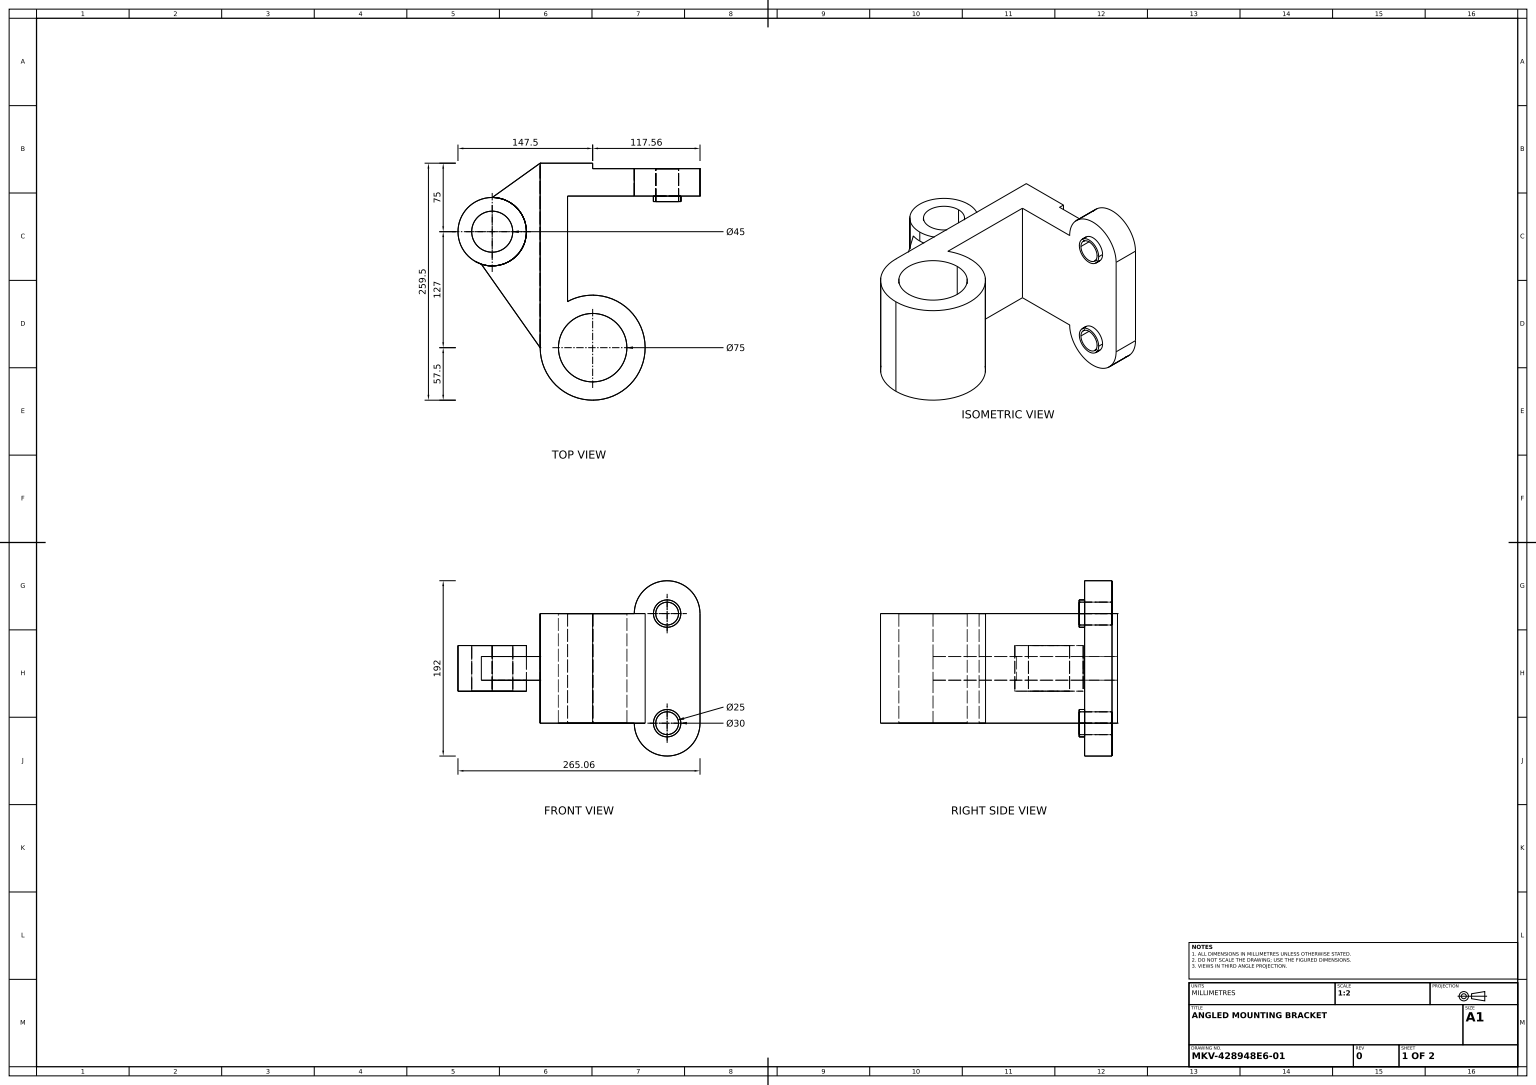
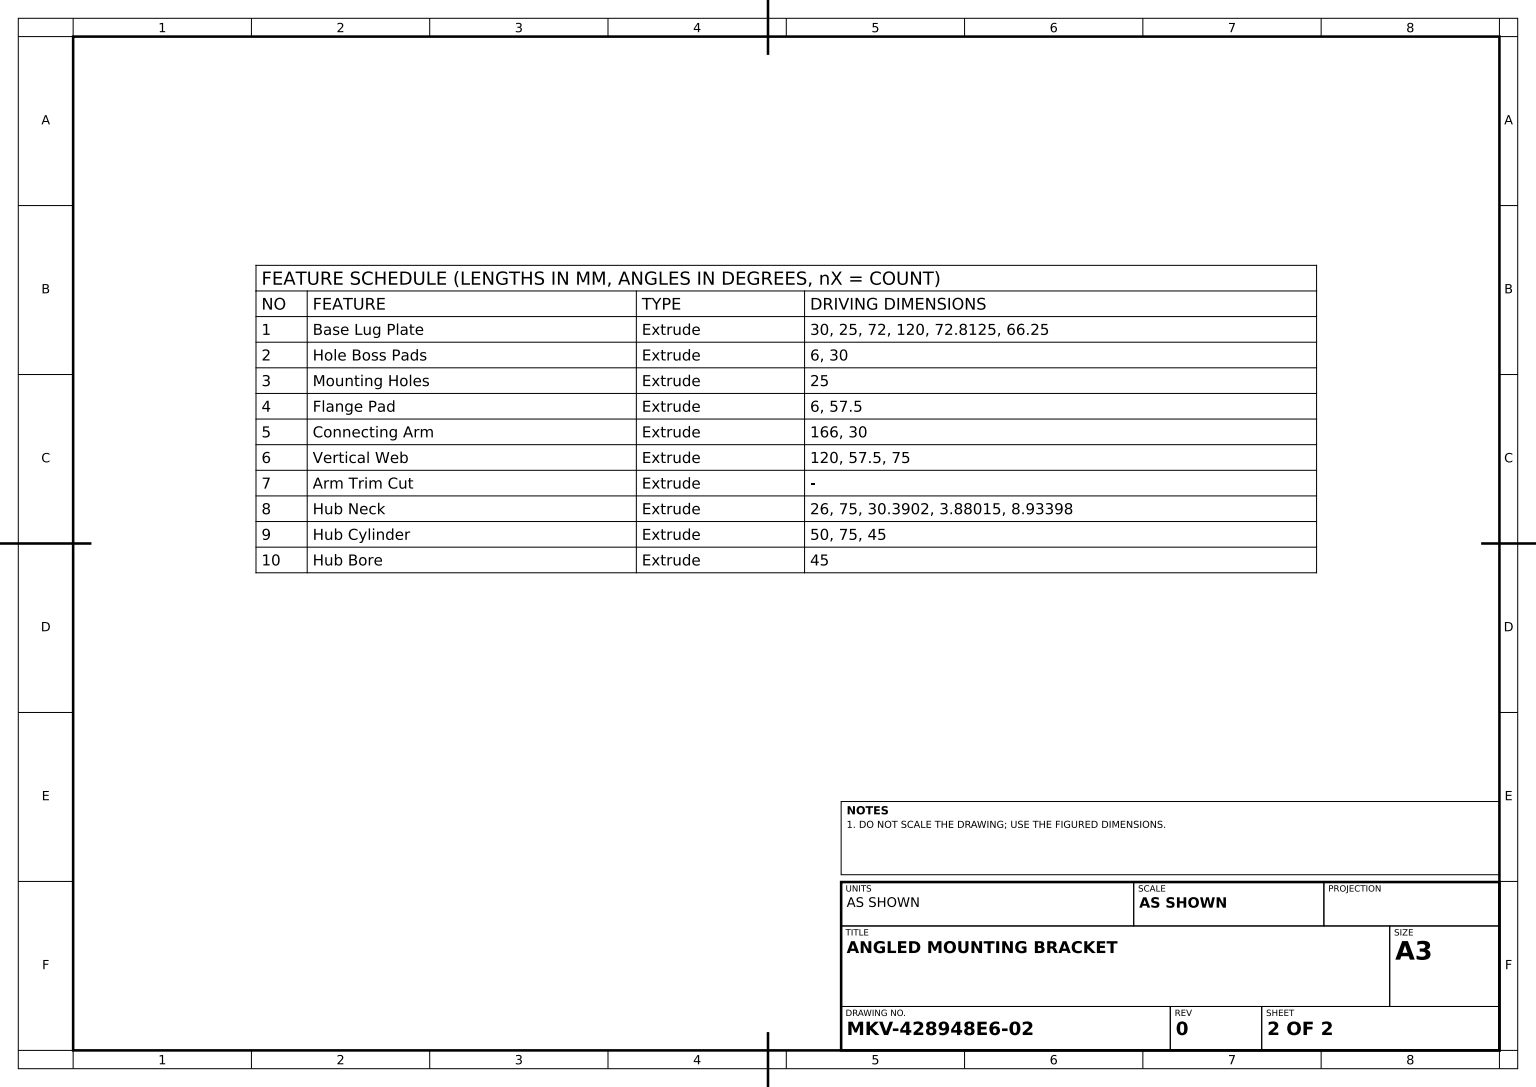
from build123d import *

# Parameters (mm, degrees)
BASE_PLATE_PROFILE_SKETCH_R = 12.5
BASE_LUG_PLATE_DEPTH        = 30
HOLE_BOSS_SKETCH_R          = 15
HOLE_BOSS_PADS_DEPTH        = 6
MOUNTING_HOLES_SKETCH_R     = 12.5
MOUNTING_HOLES_DEPTH        = 150.506388346
FLANGE_PAD_SKETCH_W         = 57.5
FLANGE_PAD_SKETCH_H         = 120
FLANGE_PAD_DEPTH            = 6
CONNECTING_ARM_SKETCH_W     = 30
CONNECTING_ARM_SKETCH_H     = 120
CONNECTING_ARM_DEPTH        = 166
VERTICAL_WEB_SKETCH_R       = 57.5
VERTICAL_WEB_SKETCH_R_2     = 37.5
VERTICAL_WEB_DEPTH          = 60
ARM_TRIM_CUT_DEPTH          = 317.920195248
HUB_NECK_DEPTH              = 13
HUB_CYLINDER_SKETCH_R       = 37.5
HUB_CYLINDER_SKETCH_R_2     = 22.5
HUB_CYLINDER_DEPTH          = 25
HUB_BORE_SKETCH_R           = 22.5
HUB_BORE_DEPTH              = 318.107730117


with BuildPart() as part:
    # Base Plate Profile Sketch → Base Lug Plate (new body)
    with BuildSketch(Plane.XY):
        with BuildLine():
            Line((108.8125, 60), (108.8125, -60))
            ThreePointArc((108.8125, -60), (72.8125, -96), (36.8125, -60))
            Line((36.8125, -60), (-66.25, -60))
            Line((-66.25, -60), (-66.25, 60))
            Line((-66.25, 60), (36.8125, 60))
            ThreePointArc((36.8125, 60), (72.8125, 96), (108.8125, 60))
        make_face()
        with Locations((72.8125, 60)):
            Circle(BASE_PLATE_PROFILE_SKETCH_R, mode=Mode.SUBTRACT)
        with Locations((72.8125, -60)):
            Circle(BASE_PLATE_PROFILE_SKETCH_R, mode=Mode.SUBTRACT)
    extrude(amount=BASE_LUG_PLATE_DEPTH)

    # Hole Boss Sketch → Hole Boss Pads (add)
    with BuildSketch(Plane.XY.offset(30)):
        with Locations((72.8125, 60)):
            Circle(HOLE_BOSS_SKETCH_R)
        with Locations((72.8125, -60)):
            Circle(HOLE_BOSS_SKETCH_R)
    extrude(amount=HOLE_BOSS_PADS_DEPTH)

    # Mounting Holes Sketch → Mounting Holes (cut, through all)
    with BuildSketch(Plane(origin=(0, 0, 0), x_dir=(-1, 0, 0), z_dir=(0, 0, -1))):
        with Locations((-72.8125, 60)):
            Circle(MOUNTING_HOLES_SKETCH_R)
        with Locations((-72.8125, -60)):
            Circle(MOUNTING_HOLES_SKETCH_R)
    extrude(amount=-MOUNTING_HOLES_DEPTH, mode=Mode.SUBTRACT)

    # Flange Pad Sketch → Flange Pad (add)
    with BuildSketch(Plane(origin=(0, 0, 0), x_dir=(-1, 0, 0), z_dir=(0, 0, -1))):
        with Locations((37.5, 0)):
            Rectangle(FLANGE_PAD_SKETCH_W, FLANGE_PAD_SKETCH_H)
    extrude(amount=FLANGE_PAD_DEPTH)

    # Connecting Arm Sketch → Connecting Arm (add)
    with BuildSketch(Plane.XY.offset(30)):
        with Locations((-51.25, 0)):
            Rectangle(CONNECTING_ARM_SKETCH_W, CONNECTING_ARM_SKETCH_H)
    extrude(amount=CONNECTING_ARM_DEPTH)

    # Vertical Web Sketch → Vertical Web (add, symmetric)
    with BuildSketch(Plane(origin=(0, 0, 0), x_dir=(1, 0, 0), z_dir=(0, 1, 0))):
        with Locations((-8.75, -196)):
            Circle(VERTICAL_WEB_SKETCH_R)
        with Locations((-8.75, -196)):
            Circle(VERTICAL_WEB_SKETCH_R_2, mode=Mode.SUBTRACT)
    extrude(amount=VERTICAL_WEB_DEPTH, both=True)

    # Arm Trim Sketch → Arm Trim Cut (cut, through all)
    with BuildSketch(Plane(origin=(0, 60, 0), x_dir=(1, 0, 0), z_dir=(0, 1, 0))):
        with BuildLine():
            Line((-36.25, -196), (-36.25, -170.504902432))
            ThreePointArc((-36.25, -170.504902432), (-43.660600109, -182.306936062), (-46.25, -196))
            Line((-46.25, -196), (-36.25, -196))
        make_face()
    extrude(amount=-ARM_TRIM_CUT_DEPTH, mode=Mode.SUBTRACT)

    # Hub Neck Sketch → Hub Neck (add, symmetric)
    with BuildSketch(Plane(origin=(0, 0, 0), x_dir=(1, 0, 0), z_dir=(0, 1, 0))):
        with BuildLine():
            Line((-141.503483954, -89.145484499), (-66.25, -196))
            Line((-66.25, -196), (-66.25, 6))
            Line((-66.25, 6), (-136.449661852, -44.296082333))
            ThreePointArc((-136.449661852, -44.296082333), (-148.385562866, -62.269844624), (-145.38363754, -83.635946473))
            Line((-145.38363754, -83.635946473), (-141.503483954, -89.145484499))
        make_face()
    extrude(amount=HUB_NECK_DEPTH, both=True)

    # Hub Cylinder Sketch → Hub Cylinder (add, symmetric)
    with BuildSketch(Plane(origin=(0, 0, 0), x_dir=(1, 0, 0), z_dir=(0, 1, 0))):
        with Locations(Location((-118.75, -69, 0), (0, 0, 270))):
            Circle(HUB_CYLINDER_SKETCH_R)
        with Locations(Location((-118.75, -69, 0), (0, 0, 270))):
            Circle(HUB_CYLINDER_SKETCH_R_2, mode=Mode.SUBTRACT)
    extrude(amount=HUB_CYLINDER_DEPTH, both=True)

    # Hub Bore Sketch → Hub Bore (cut, through all)
    with BuildSketch(Plane(origin=(0, 13, 0), x_dir=(1, 0, 0), z_dir=(0, 1, 0))):
        with Locations(Location((-118.75, -69, 0), (0, 0, 270))):
            Circle(HUB_BORE_SKETCH_R)
    extrude(amount=-HUB_BORE_DEPTH, mode=Mode.SUBTRACT)


solid = part.part
